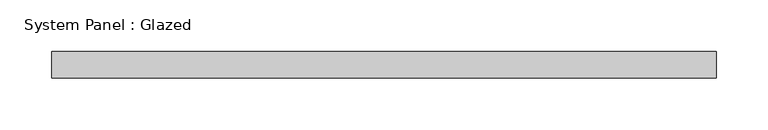
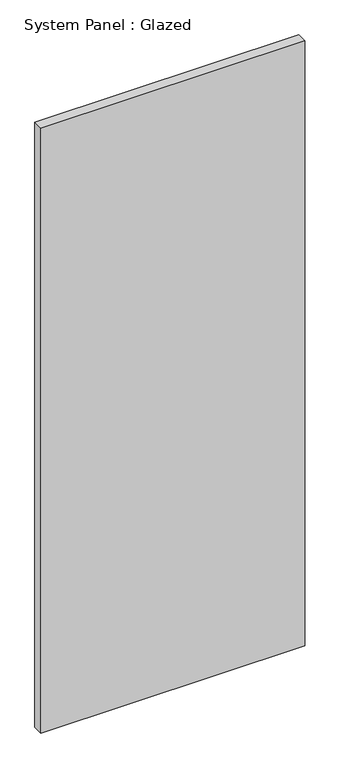
"""IFC4 building model written with IfcOpenShell, lengths in millimetres: plate geometry, System Panel : Glazed."""

from ifc_helpers import new_model, si_unit, origin, origin_with_axes, place, context, project, spatial, polyline, outline, extrude, source, transform, mapped, element, save


def system_panel_glazed_46d50955(model_context):
    return source(origin(), model_context, "Body", "SweptSolid", [
        extrude(outline(polyline([(320.675, 19.05), (-320.675, 19.05), (-320.675, 44.45), (320.675, 44.45), (320.675, 19.05)])), origin_with_axes(), (0.0, 0.0, 1.0), 1555.0744644),
    ])


if __name__ == "__main__":
    model = new_model("IFC4")
    model_context = context("Model", 3, world=origin())
    ifc_project = project(units=[si_unit("LENGTHUNIT", "METRE", prefix="MILLI")], contexts=[model_context])
    site = spatial("IfcSite", under=ifc_project)
    building = spatial("IfcBuilding", under=site)
    placement = place(None, origin())
    system_panel_glazed_shape = system_panel_glazed_46d50955(model_context)
    element("IfcPlate", 1, ObjectType="System Panel : Glazed", at=placement, inside=building, context=model_context, shape_type="MappedRepresentation", body=[
        mapped(system_panel_glazed_shape, transform((0.0, 0.0, 0.0), x_axis=(1.0, 0.0, 0.0), y_axis=(0.0, 1.0, 0.0), z_axis=(0.0, 0.0, 1.0))),
    ])
    save(model, "model.ifc")

# Revit data of these elements
# Type "System Panel : Glazed"
#   Construction Type Id = "GSP4R"
#   Analytic Construction = "1/8 in Pilkington single glazing"
#   Visual Light Transmittance = 0.9
#   Solar Heat Gain Coefficient = 0.86
#   Heat Transfer Coefficient (U) = 1.18115 BTU/(h·ft²·°F)
#   Define Thermal Properties by = 1
# Element 1 (IfcPlate, "System Panel : Glazed")
#   Materials on its faces: "Glass"
# Materials
#   "Glass": class "Glass", colour RGB 0 128 192, transparency 0.75, Description = "Soda Lime Glass", Cost = 0
